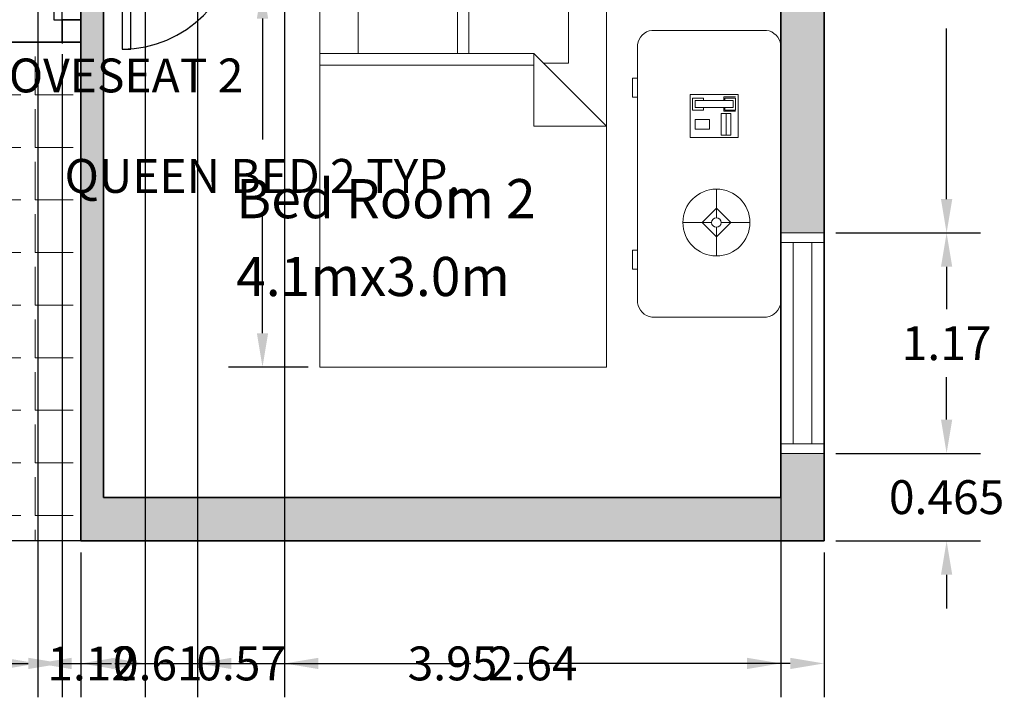
# Model space of a CAD drawing. Units: metres. Extents: x 35.2 to 46.4, y 446.1 to 460.8.
# Tile 2 of 6: x 40.7 to 45.9, y 446.1 to 449.7. Entities that reach past the tile are written whole.
import ezdxf

# ---------------------------------------------------------------- set-up
doc = ezdxf.new("R2010")
doc.units = ezdxf.units.M
for name, color, linetype, lineweight in [('A-ANNO-DIMS', 2, 'Continuous', 18), ('A-AREA-IDEN', 7, 'Continuous', 18), ('A-DOOR', 3, 'Continuous', 25), ('A-EQPM', 8, 'Continuous', 13), ('A-FLOR', 7, 'Continuous', 25), ('A-FLOR-PATT', 9, 'Continuous', 13), ('A-GLAZ', 4, 'Continuous', 18), ('A-WALL', 7, 'Continuous', 35), ('A-WALL-PATT', 252, 'Continuous', 13), ('FURNITURE', 53, 'Continuous', 18)]:
    doc.layers.add(name, color=color, linetype=linetype, lineweight=lineweight)
doc.styles.get("Standard").update_dxf_attribs({"font": 'calibri.ttf'})
doc.dimstyles.get("Standard").update_dxf_attribs({"dimtxt": 0.18, "dimasz": 0.18, "dimexe": 0.18, "dimexo": 0.0625, "dimgap": 0.09, "dimtad": 0, "dimtih": 1, "dimtoh": 1, "dimdec": 4, "dimzin": 0, "dimdsep": 46, "dimtxsty": 'Standard', "dimcen": 0.09, "dimadec": 0, "dimazin": 0, "dimtfac": 1, "dimtdec": 4, "dimtofl": 0, "dimtmove": 0, "dimatfit": 3, "dimfxl": 1, "dimtolj": 1, "dimtzin": 0, "dimarcsym": 0})

# ---------------------------------------------------------------- blocks, each defined once
blk = doc.blocks.new('*U3')
for p, q in [((0, 0), (0, 5)), ((24, 0), (24, 5))]:
    blk.add_line(p, q)
blk.add_lwpolyline([(0, 0), (0, -24), (1.75, -24), (1.75, 0)], close=True)
blk.add_arc((0, 0), 24, 270, 0)
blk = doc.blocks.new('*U4')
for p, q in [((-24, 0), (-24, -5)), ((0, 0), (0, -5))]:
    blk.add_line(p, q)
blk.add_lwpolyline([(0, 0), (0, 24), (-1.75, 24), (-1.75, 0)], close=True)
blk.add_arc((0, 0), 24, 90, 180)
blk = doc.blocks.new('Bed - Queen')
for p, q in [((0, -80.00003), (0, 0)), ((0, 0), (59.99999, 0)), ((59.99999, 0), (59.99999, -80.00003)), ((7.99999, -1.2), (28.79998, -1.2)), ((7.99999, -14.4), (7.99999, -1.2)), ((28.79998, -1.2), (28.79998, -14.4)), ((31.19999, -1.2), (51.99999, -1.2)), ((31.19999, -14.4), (31.19999, -1.2)), ((51.99999, -1.2), (51.99999, -16.4)), ((0, -14.4), (44.8, -14.4)), ((59.99999, -29.6), (44.8, -14.4)), ((44.8, -14.4), (44.8, -29.6)), ((51.99999, -16.4), (46.79936, -16.4)), ((44.8, -16.8), (0, -16.8)), ((44.8, -29.6), (59.99999, -29.6)), ((59.99999, -80.00003), (0, -80.00003))]:
    blk.add_line(p, q)
blk = doc.blocks.new('Desk - 30 x 60 in.')
for p, q in [((-26.999995, 0), (26.999995, 0)), ((-29.999995, -27), (-29.999995, -3)), ((29.999995, -3), (29.999995, -27)), ((26.999995, -30), (-26.999995, -30)), ((-20.000005, -30), (-20.000005, -31)), ((-16.000005, -31), (-16.000005, -30)), ((15.999995, -31), (15.999995, -30)), ((19.999995, -30), (19.999995, -31)), ((-20.000005, -31), (-16.000005, -31)), ((19.999995, -31), (15.999995, -31))]:
    blk.add_line(p, q)
for centre, start, end in [((-26.499995, -3.5), 98.1301, 171.8699), ((26.499995, -3.5), 8.130102, 81.8699), ((-26.499995, -26.5), 188.1301, 261.8699), ((26.499995, -26.5), 278.1301, 351.8699)]:
    blk.add_arc(centre, 3.535534, start, end)
blk = doc.blocks.new('Lamp - Table')
for p, q in [((0, 7), (0, 1)), ((0, 3), (-3, 0)), ((3, 0), (0, 3)), ((-1, 0), (-7, 0)), ((-3, 0), (0, -3)), ((0, -3), (3, 0)), ((1, 0), (7, 0)), ((0, -1), (0, -7))]:
    blk.add_line(p, q)
for radius in [7, 1]:
    blk.add_circle((0, 0), radius)
blk = doc.blocks.new('Phone - Desk')
for p, q in [((-4.5, -5), (-4.5, 5)), ((-4.5, 5), (4.5, 5)), ((-4, 4.5), (-4, 2)), ((-3.75, 4.5), (-3.75, 2.25)), ((-1.25, 4.5), (-3.75, 4.5)), ((-1.25, 2.25), (-1.25, 4.5)), ((-1, 2), (-1, 4.5)), ((4.5, 5), (4.5, -5)), ((-3.75, 2.25), (-3.25, 2.25)), ((-3.25, 4), (-3.25, -4)), ((-3.25, 4), (-1.75, 4)), ((-1.75, -4), (-1.75, 4)), ((-1.75, 2.25), (-1.25, 2.25)), ((4, 3.5), (-0.5, 3.5)), ((-0.5, 3.5), (-0.5, 1.5)), ((-0.5, 2.5), (4, 2.5)), ((4, 1.5), (4, 3.5)), ((-4, 2), (-3.25, 2)), ((-1.75, 2), (-1, 2)), ((-0.5, 1.5), (4, 1.5)), ((2.75, -1), (0.75, -1)), ((0.75, -1), (0.75, -4)), ((2.75, -4), (2.75, -1)), ((-3.75, -2.25), (-3.25, -2.25)), ((-3.75, -4.5), (-3.75, -2.25)), ((-3.25, -4), (-1.75, -4)), ((-1.75, -2.25), (-1.25, -2.25)), ((-1.25, -2.25), (-1.25, -4.5)), ((0.75, -4), (2.75, -4)), ((4.5, -5), (-4.5, -5)), ((-1.25, -4.5), (-3.75, -4.5))]:
    blk.add_line(p, q)
blk = doc.blocks.new('WIN-1172')
for p, q in [((0, 1.1716), (0.23, 1.1716)), ((0, 1.1716), (0, 0)), ((0.23, 1.1716), (0.23, 0)), ((0, 1.1216), (0.23, 1.1216)), ((0.065, 1.1216), (0.065, 0.05)), ((0.165, 1.1216), (0.165, 0.05)), ((0.23, 0.05), (0, 0.05)), ((0.23, 0), (0, 0))]:
    blk.add_line(p, q)
blk = doc.blocks.new('*D131')
at = {"layer": 'A-ANNO-DIMS', "color": 0, "lineweight": -2, "transparency": 16777216}
for p, q in [((42.244, 449.8606), (41.8217, 449.8606)), ((42.0017, 449.6806), (42.0017, 449.0387)), ((42.0017, 448.0086), (42.0017, 448.6505)), ((42.244, 447.8286), (41.8217, 447.8286))]:
    blk.add_line(p, q, dxfattribs=at)
at = {"layer": 'A-ANNO-DIMS', "color": 0, "transparency": 16777216}
for points in [[(41.9717, 449.6806), (42.0317, 449.6806), (42.0017, 449.8606)], [(41.9717, 448.0086), (42.0317, 448.0086), (42.0017, 447.8286)]]:
    blk.add_solid(points, dxfattribs=at)
at = {"layer": 'Defpoints', "color": 0, "transparency": 16777216}
for p in [(42.0017, 449.8606), (42.3065, 449.8606), (42.3065, 447.8286)]:
    blk.add_point(p, dxfattribs=at)
at = {"layer": 'A-ANNO-DIMS', "color": 0, "transparency": 16777216, "insert": (42.0017, 448.8446), "char_height": 0.18, "attachment_point": 5}
blk.add_mtext('\\A1;QUEEN BED 2 TYP.', dxfattribs=at)
blk = doc.blocks.new('*D147')
at = {"layer": 'A-ANNO-DIMS', "color": 0, "lineweight": -2, "transparency": 16777216}
for p, q in [((38.7435, 449.5445), (38.7435, 449.1984)), ((40.2675, 449.5445), (40.2675, 449.1984)), ((38.9235, 449.3784), (40.0875, 449.3784)), ((40.2675, 449.3784), (40.4475, 449.3784))]:
    blk.add_line(p, q, dxfattribs=at)
at = {"layer": 'A-ANNO-DIMS', "color": 0, "transparency": 16777216}
for points in [[(38.9235, 449.4084), (38.9235, 449.3484), (38.7435, 449.3784)], [(40.0875, 449.4084), (40.0875, 449.3484), (40.2675, 449.3784)]]:
    blk.add_solid(points, dxfattribs=at)
at = {"layer": 'Defpoints', "color": 0, "transparency": 16777216}
for p in [(38.7435, 449.607), (40.2675, 449.607), (40.2675, 449.3784)]:
    blk.add_point(p, dxfattribs=at)
at = {"layer": 'A-ANNO-DIMS', "color": 0, "transparency": 16777216, "insert": (41.2103, 449.3784), "char_height": 0.18, "attachment_point": 5}
blk.add_mtext('\\A1;LOVESEAT 2', dxfattribs=at)
blk = doc.blocks.new('*D153')
at = {"layer": 'A-ANNO-DIMS', "color": 0, "lineweight": -2, "transparency": 16777216}
for p, q in [((41.0366, 446.8423), (41.0366, 446.0736)), ((44.9866, 446.8423), (44.9866, 446.0736)), ((41.2166, 446.2536), (42.6857, 446.2536)), ((44.8066, 446.2536), (43.3375, 446.2536))]:
    blk.add_line(p, q, dxfattribs=at)
at = {"layer": 'A-ANNO-DIMS', "color": 0, "transparency": 16777216}
for points in [[(41.2166, 446.2836), (41.2166, 446.2236), (41.0366, 446.2536)], [(44.8066, 446.2836), (44.8066, 446.2236), (44.9866, 446.2536)]]:
    blk.add_solid(points, dxfattribs=at)
at = {"layer": 'Defpoints', "color": 0, "transparency": 16777216}
for p in [(41.0366, 446.9048), (44.9866, 446.9048), (44.9866, 446.2536)]:
    blk.add_point(p, dxfattribs=at)
at = {"layer": 'A-ANNO-DIMS', "color": 0, "transparency": 16777216, "insert": (43.0116, 446.2536), "char_height": 0.18, "attachment_point": 5}
blk.add_mtext('\\A1;3.95', dxfattribs=at)
blk = doc.blocks.new('*D154')
at = {"layer": 'A-ANNO-DIMS', "color": 0, "lineweight": -2, "transparency": 16777216}
for p, q in [((40.9741, 449.5548), (40.2054, 449.5548)), ((40.3854, 449.3748), (40.3854, 448.412)), ((40.3854, 447.0848), (40.3854, 448.0476)), ((40.9741, 446.9048), (40.2054, 446.9048))]:
    blk.add_line(p, q, dxfattribs=at)
at = {"layer": 'A-ANNO-DIMS', "color": 0, "transparency": 16777216}
for points in [[(40.3554, 449.3748), (40.4154, 449.3748), (40.3854, 449.5548)], [(40.3554, 447.0848), (40.4154, 447.0848), (40.3854, 446.9048)]]:
    blk.add_solid(points, dxfattribs=at)
at = {"layer": 'Defpoints', "color": 0, "transparency": 16777216}
for p in [(40.3854, 449.5548), (41.0366, 449.5548), (41.0366, 446.9048)]:
    blk.add_point(p, dxfattribs=at)
at = {"layer": 'A-ANNO-DIMS', "color": 0, "transparency": 16777216, "insert": (40.3854, 448.2298), "char_height": 0.18, "attachment_point": 5}
blk.add_mtext('\\A1;2.65', dxfattribs=at)
blk = doc.blocks.new('*D159')
at = {"layer": 'A-ANNO-DIMS', "color": 0, "lineweight": -2, "transparency": 16777216}
for p, q in [((45.637795, 447.549797), (45.637795, 447.729797)), ((45.049095, 447.369797), (45.817795, 447.369797)), ((45.049095, 446.904779), (45.817795, 446.904779)), ((45.637795, 446.724779), (45.637795, 446.544779))]:
    blk.add_line(p, q, dxfattribs=at)
at = {"layer": 'A-ANNO-DIMS', "color": 0, "transparency": 16777216}
for points in [[(45.607795, 447.549797), (45.667795, 447.549797), (45.637795, 447.369797)], [(45.607795, 446.724779), (45.667795, 446.724779), (45.637795, 446.904779)]]:
    blk.add_solid(points, dxfattribs=at)
at = {"layer": 'Defpoints', "color": 0, "transparency": 16777216}
for p in [(44.986595, 447.369797), (45.637795, 447.369797), (44.986595, 446.904779)]:
    blk.add_point(p, dxfattribs=at)
at = {"layer": 'A-ANNO-DIMS', "color": 0, "transparency": 16777216, "insert": (45.637795, 447.137288), "char_height": 0.18, "attachment_point": 5}
blk.add_mtext('\\A1;0.465', dxfattribs=at)
blk = doc.blocks.new('*D160')
at = {"layer": 'A-ANNO-DIMS', "color": 0, "lineweight": -2, "transparency": 16777216}
for p, q in [((45.0491, 448.5414), (45.8178, 448.5414)), ((45.6378, 448.3614), (45.6378, 448.1364)), ((45.6378, 447.5498), (45.6378, 447.7747)), ((45.0491, 447.3698), (45.8178, 447.3698))]:
    blk.add_line(p, q, dxfattribs=at)
at = {"layer": 'A-ANNO-DIMS', "color": 0, "transparency": 16777216}
for points in [[(45.6078, 448.3614), (45.6678, 448.3614), (45.6378, 448.5414)], [(45.6078, 447.5498), (45.6678, 447.5498), (45.6378, 447.3698)]]:
    blk.add_solid(points, dxfattribs=at)
at = {"layer": 'Defpoints', "color": 0, "transparency": 16777216}
for p in [(44.9866, 448.5414), (45.6378, 448.5414), (44.9866, 447.3698)]:
    blk.add_point(p, dxfattribs=at)
at = {"layer": 'A-ANNO-DIMS', "color": 0, "transparency": 16777216, "insert": (45.6378, 447.9556), "char_height": 0.18, "attachment_point": 5}
blk.add_mtext('\\A1;1.17', dxfattribs=at)
blk = doc.blocks.new('*D161')
at = {"layer": 'A-ANNO-DIMS', "color": 0, "lineweight": -2, "transparency": 16777216}
for p, q in [((45.0491, 451.0803), (45.8178, 451.0803)), ((45.6378, 450.9003), (45.6378, 449.9931)), ((45.6378, 448.7214), (45.6378, 449.6286)), ((45.0491, 448.5414), (45.8178, 448.5414))]:
    blk.add_line(p, q, dxfattribs=at)
at = {"layer": 'A-ANNO-DIMS', "color": 0, "transparency": 16777216}
for points in [[(45.6078, 450.9003), (45.6678, 450.9003), (45.6378, 451.0803)], [(45.6078, 448.7214), (45.6678, 448.7214), (45.6378, 448.5414)]]:
    blk.add_solid(points, dxfattribs=at)
at = {"layer": 'Defpoints', "color": 0, "transparency": 16777216}
for p in [(44.9866, 451.0803), (45.6378, 451.0803), (44.9866, 448.5414)]:
    blk.add_point(p, dxfattribs=at)
at = {"layer": 'A-ANNO-DIMS', "color": 0, "transparency": 16777216, "insert": (45.6378, 449.8109), "char_height": 0.18, "attachment_point": 5}
blk.add_mtext('\\A1;2.539', dxfattribs=at)
blk = doc.blocks.new('*D167')
at = {"layer": 'A-ANNO-DIMS', "color": 0, "lineweight": -2, "transparency": 16777216}
for p, q in [((37.8366, 459.6323), (37.8366, 446.0736)), ((40.8069, 459.6323), (40.8069, 446.0736)), ((38.0166, 446.2536), (38.9948, 446.2536)), ((40.6269, 446.2536), (39.6486, 446.2536))]:
    blk.add_line(p, q, dxfattribs=at)
at = {"layer": 'A-ANNO-DIMS', "color": 0, "transparency": 16777216}
for points in [[(38.0166, 446.2836), (38.0166, 446.2236), (37.8366, 446.2536)], [(40.6269, 446.2836), (40.6269, 446.2236), (40.8069, 446.2536)]]:
    blk.add_solid(points, dxfattribs=at)
at = {"layer": 'Defpoints', "color": 0, "transparency": 16777216}
for p in [(37.8366, 459.6948), (40.8069, 459.6948), (40.8069, 446.2536)]:
    blk.add_point(p, dxfattribs=at)
at = {"layer": 'A-ANNO-DIMS', "color": 0, "transparency": 16777216, "insert": (39.3217, 446.2536), "char_height": 0.18, "attachment_point": 5}
blk.add_mtext('\\A1;2.97', dxfattribs=at)
blk = doc.blocks.new('*D168')
at = {"layer": 'A-ANNO-DIMS', "color": 0, "lineweight": -2, "transparency": 16777216}
for p, q in [((40.8069, 459.6323), (40.8069, 446.0736)), ((41.3784, 459.6323), (41.3784, 446.0736)), ((40.9869, 446.2536), (41.1984, 446.2536)), ((41.3784, 446.2536), (41.5584, 446.2536))]:
    blk.add_line(p, q, dxfattribs=at)
at = {"layer": 'A-ANNO-DIMS', "color": 0, "transparency": 16777216}
for points in [[(40.9869, 446.2836), (40.9869, 446.2236), (40.8069, 446.2536)], [(41.1984, 446.2836), (41.1984, 446.2236), (41.3784, 446.2536)]]:
    blk.add_solid(points, dxfattribs=at)
at = {"layer": 'Defpoints', "color": 0, "transparency": 16777216}
for p in [(40.8069, 459.6948), (41.3784, 459.6948), (41.3784, 446.2536)]:
    blk.add_point(p, dxfattribs=at)
at = {"layer": 'A-ANNO-DIMS', "color": 0, "transparency": 16777216, "insert": (41.8883, 446.2536), "char_height": 0.18, "attachment_point": 5}
blk.add_mtext('\\A1;0.57', dxfattribs=at)
blk = doc.blocks.new('*D169')
at = {"layer": 'A-ANNO-DIMS', "color": 0, "lineweight": -2, "transparency": 16777216}
for p, q in [((40.536595, 457.132279), (40.536595, 446.073579)), ((41.656595, 457.132279), (41.656595, 446.073579)), ((40.356595, 446.253579), (40.176595, 446.253579)), ((41.836595, 446.253579), (42.016595, 446.253579))]:
    blk.add_line(p, q, dxfattribs=at)
at = {"layer": 'A-ANNO-DIMS', "color": 0, "transparency": 16777216}
for points in [[(40.356595, 446.283579), (40.356595, 446.223579), (40.536595, 446.253579)], [(41.836595, 446.283579), (41.836595, 446.223579), (41.656595, 446.253579)]]:
    blk.add_solid(points, dxfattribs=at)
at = {"layer": 'Defpoints', "color": 0, "transparency": 16777216}
for p in [(40.536595, 457.194779), (41.656595, 457.194779), (41.656595, 446.253579)]:
    blk.add_point(p, dxfattribs=at)
at = {"layer": 'A-ANNO-DIMS', "color": 0, "transparency": 16777216, "insert": (41.096595, 446.253579), "char_height": 0.18, "attachment_point": 5}
blk.add_mtext('\\A1;1.12', dxfattribs=at)
blk = doc.blocks.new('*D171')
at = {"layer": 'A-ANNO-DIMS', "color": 0, "lineweight": -2, "transparency": 16777216}
for p, q in [((42.1191, 450.1923), (42.1191, 446.0736)), ((44.7566, 450.1923), (44.7566, 446.0736)), ((42.2991, 446.2536), (43.1085, 446.2536)), ((44.5766, 446.2536), (43.7673, 446.2536))]:
    blk.add_line(p, q, dxfattribs=at)
at = {"layer": 'A-ANNO-DIMS', "color": 0, "transparency": 16777216}
for points in [[(42.2991, 446.2836), (42.2991, 446.2236), (42.1191, 446.2536)], [(44.5766, 446.2836), (44.5766, 446.2236), (44.7566, 446.2536)]]:
    blk.add_solid(points, dxfattribs=at)
at = {"layer": 'Defpoints', "color": 0, "transparency": 16777216}
for p in [(42.1191, 450.2548), (44.7566, 450.2548), (44.7566, 446.2536)]:
    blk.add_point(p, dxfattribs=at)
at = {"layer": 'A-ANNO-DIMS', "color": 0, "transparency": 16777216, "insert": (43.4379, 446.2536), "char_height": 0.18, "attachment_point": 5}
blk.add_mtext('\\A1;2.64', dxfattribs=at)
blk = doc.blocks.new('*D174')
at = {"layer": 'A-ANNO-DIMS', "color": 0, "lineweight": -2, "transparency": 16777216}
for p, q in [((40.327, 449.4923), (40.327, 446.0736)), ((40.9366, 449.4923), (40.9366, 446.0736)), ((40.507, 446.2536), (40.7566, 446.2536)), ((40.9366, 446.2536), (41.1166, 446.2536))]:
    blk.add_line(p, q, dxfattribs=at)
at = {"layer": 'A-ANNO-DIMS', "color": 0, "transparency": 16777216}
for points in [[(40.507, 446.2836), (40.507, 446.2236), (40.327, 446.2536)], [(40.7566, 446.2836), (40.7566, 446.2236), (40.9366, 446.2536)]]:
    blk.add_solid(points, dxfattribs=at)
at = {"layer": 'Defpoints', "color": 0, "transparency": 16777216}
for p in [(40.327, 449.5548), (40.9366, 449.5548), (40.9366, 446.2536)]:
    blk.add_point(p, dxfattribs=at)
at = {"layer": 'A-ANNO-DIMS', "color": 0, "transparency": 16777216, "insert": (41.4453, 446.2536), "char_height": 0.18, "attachment_point": 5}
blk.add_mtext('\\A1;0.61', dxfattribs=at)

msp = doc.modelspace()

# ---------------------------------------------------------------- hatches: boundary and pattern name
at = {"layer": 'A-FLOR-PATT'}
h = msp.add_hatch(dxfattribs=at)
h.set_pattern_fill('ANGLE', color=256, scale=0.04)
h.set_pattern_definition([(0, (0, 0), (0, 0.2794), [0.2032, -0.0762]), (90, (0, 0), (-0.2794, 0), [0.2032, -0.0762])])
h.paths.add_polyline_path([(41.0366, 449.5548), (37.6066, 449.5548), (37.6066, 446.9048), (41.0366, 446.9048)])
at = {"layer": 'A-WALL-PATT'}
h = msp.add_hatch(color=256, dxfattribs=at)
h.dxf.hatch_style = 1
h.paths.add_polyline_path([(44.9866, 457.1611), (44.7566, 457.1611), (44.7566, 454.5208), (44.9866, 454.5208)])
h.paths.add_polyline_path([(44.9866, 453.3493), (44.7566, 453.3493), (44.7566, 452.3748), (42.8766, 452.3748), (42.8766, 452.8748), (42.1191, 452.8748), (42.1191, 452.9307), (41.9991, 452.9307), (41.9991, 452.2548), (42.1191, 452.2548), (42.1191, 452.7548), (42.7566, 452.7548), (42.7566, 452.2548), (44.7566, 452.2548), (44.7566, 451.6519), (44.9866, 451.6519)])
h.paths.add_polyline_path([(44.9866, 451.0803), (44.7566, 451.0803), (44.7566, 450.2548), (43.6593, 450.2548), (43.0598, 450.2548, -0.016107), (43.0354, 450.2548), (42.1191, 450.2548), (42.1191, 450.7446), (41.9991, 450.7446), (41.9991, 450.2548), (41.8662, 450.2548), (41.8662, 450.1348), (44.7566, 450.1348), (44.7566, 448.5414), (44.9866, 448.5414)])
h.paths.add_polyline_path([(44.9866, 447.3698), (44.7566, 447.3698), (44.7566, 447.1348), (41.1566, 447.1348), (41.1566, 450.1348), (41.2566, 450.1348), (41.2566, 450.2548), (41.0366, 450.2548), (41.0366, 446.9048), (44.9866, 446.9048)])

# ---------------------------------------------------------------- linework, layer by layer
at = {"layer": 'A-FLOR'}
msp.add_lwpolyline([(37.6066, 449.5548), (41.0366, 449.5548), (41.0366, 446.9048), (37.6066, 446.9048)], close=True, dxfattribs=at)
at = {"layer": 'A-WALL'}
for p, q in [((44.9866, 459.9248), (44.9866, 446.9048)), ((41.0366, 450.2548), (41.0366, 446.9048)), ((41.1566, 450.1348), (41.1566, 447.1348)), ((44.7566, 450.1348), (44.7566, 447.1348)), ((40.9366, 449.6748), (40.9366, 449.5548)), ((40.9366, 449.6748), (41.0366, 449.6748)), ((40.9366, 449.5548), (41.0366, 449.5548)), ((41.1566, 447.1348), (44.7566, 447.1348)), ((41.0366, 446.9048), (44.9866, 446.9048))]:
    msp.add_line(p, q, dxfattribs=at)

# ---------------------------------------------------------------- block references
at = {"layer": 'A-DOOR', "xscale": 0.0254, "yscale": 0.0254, "zscale": 0.0254}
for name, p in [('*U4', (40.9366, 449.6748)), ('*U3', (41.2566, 450.1278))]:
    msp.add_blockref(name, p, dxfattribs=at)
at = {"layer": 'A-EQPM', "transparency": 33554521, "xscale": 0.0254, "yscale": 0.0254, "zscale": 0.0254, "rotation": 270}
for name, p in [('Phone - Desk', (44.4022, 449.163)), ('Lamp - Table', (44.4142, 448.5968))]:
    msp.add_blockref(name, p, dxfattribs=at)
at = {"layer": 'A-GLAZ'}
msp.add_blockref('WIN-1172', (44.7566, 447.3698), dxfattribs=at)
at = {"layer": 'FURNITURE', "transparency": 33554521, "xscale": 0.0254, "yscale": 0.0254, "zscale": 0.0254}
msp.add_blockref('Bed - Queen', (42.3065, 449.8606), dxfattribs=at)
at = {"layer": 'FURNITURE', "transparency": 33554521, "xscale": 0.0254, "yscale": 0.0254, "zscale": 0.0254, "rotation": 270}
msp.add_blockref('Desk - 30 x 60 in.', (44.7566, 448.8562), dxfattribs=at)

# ---------------------------------------------------------------- texts
at = {"layer": 'A-AREA-IDEN'}
for s, p in [('Bed Room 2', (41.8616, 448.6196)), ('4.1mx3.0m', (41.8616, 448.206))]:
    msp.add_text(s, height=0.20807, dxfattribs=at).set_placement(p)

# ---------------------------------------------------------------- dimensions: what is measured, and where the dimension line sits
at = {"layer": 'A-ANNO-DIMS'}
for base, p1, p2, picture, middle in [((40.8069, 446.2536), (37.8366, 459.6948), (40.8069, 459.6948), '*D167', (39.3217, 446.2536)), ((41.3784, 446.2536), (40.8069, 459.6948), (41.3784, 459.6948), '*D168', (41.8883, 446.2536)), ((41.6566, 446.2536), (40.5366, 457.1948), (41.6566, 457.1948), '*D169', (41.0966, 446.2536)), ((44.7566, 446.2536), (42.1191, 450.2548), (44.7566, 450.2548), '*D171', (43.4379, 446.2536)), ((40.9366, 446.2536), (40.327, 449.5548), (40.9366, 449.5548), '*D174', (41.4453, 446.2536)), ((44.9866, 446.2536), (41.0366, 446.9048), (44.9866, 446.9048), '*D153', (43.0116, 446.2536))]:
    dim = msp.add_linear_dim(base=base, p1=p1, p2=p2, dimstyle='Standard', override={"dimdec": 2, "dimlfac": 1, "dimrnd": 0, "dimzin": 0, "dimdsep": 46, "dimlunit": 2}, dxfattribs=at)
    dim.commit()
    dim.dimension.update_dxf_attribs({"geometry": picture, "text_midpoint": middle})
for base, p1, p2, override, picture, middle in [((45.6378, 451.0803), (44.9866, 448.5414), (44.9866, 451.0803), {"dimdec": 3, "dimlfac": 1, "dimrnd": 0, "dimzin": 0, "dimdsep": 46, "dimlunit": 2}, '*D161', (45.6378, 449.8109)), ((40.3854, 449.5548), (41.0366, 446.9048), (41.0366, 449.5548), {"dimdec": 2, "dimlfac": 1, "dimrnd": 0, "dimzin": 0, "dimdsep": 46, "dimlunit": 2}, '*D154', (40.3854, 448.2298)), ((45.6378, 448.5414), (44.9866, 447.3698), (44.9866, 448.5414), {"dimdec": 2, "dimlfac": 1, "dimrnd": 0, "dimzin": 0, "dimdsep": 46, "dimlunit": 2}, '*D160', (45.6378, 447.9556)), ((45.6378, 447.3698), (44.9866, 446.9048), (44.9866, 447.3698), {"dimdec": 3, "dimlfac": 1, "dimrnd": 0, "dimzin": 0, "dimdsep": 46, "dimlunit": 2}, '*D159', (45.6378, 447.1373))]:
    dim = msp.add_linear_dim(base=base, p1=p1, p2=p2, angle=90, dimstyle='Standard', override=override, dxfattribs=at)
    dim.commit()
    dim.dimension.update_dxf_attribs({"geometry": picture, "text_midpoint": middle})
dim = msp.add_linear_dim(base=(42.0017, 449.8606), p1=(42.3065, 447.8286), p2=(42.3065, 449.8606), angle=90, text='QUEEN BED <> TYP.', dimstyle='Standard', override={"dimdec": 0, "dimlfac": 1, "dimrnd": 0, "dimzin": 0, "dimdsep": 46, "dimlunit": 2}, dxfattribs=at)
dim.commit()
dim.dimension.update_dxf_attribs({"geometry": '*D131', "text_midpoint": (42.0017, 448.8446)})
dim = msp.add_linear_dim(base=(40.2675, 449.3784), p1=(38.7435, 449.607), p2=(40.2675, 449.607), text='LOVESEAT <>', dimstyle='Standard', override={"dimdec": 0, "dimlfac": 1, "dimrnd": 0, "dimzin": 0, "dimdsep": 46, "dimlunit": 2}, dxfattribs=at)
dim.commit()
dim.dimension.update_dxf_attribs({"geometry": '*D147', "text_midpoint": (41.2103, 449.3784)})

doc.saveas('drawing.dxf')
